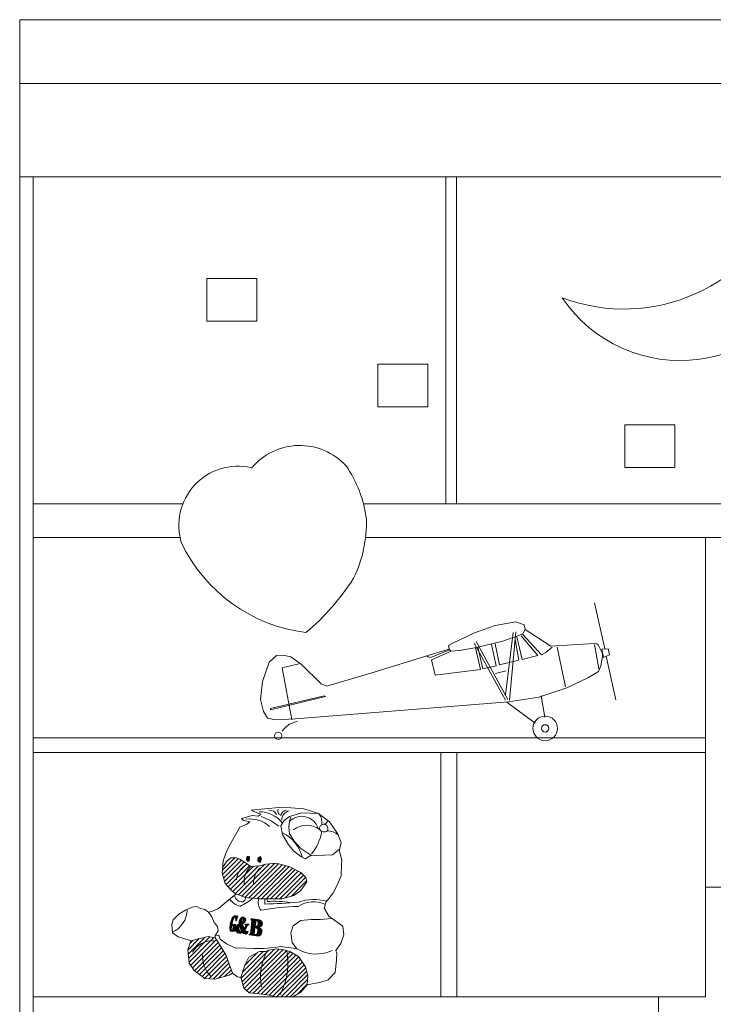
# Model space of a CAD drawing. Units: inches. Extents: x -17 to 1735, y -531 to 60.
# Tile 18 of 27: x 1734.74915 to 1734.79189, y -150.22283 to -150.1622. Entities that reach past the tile are written whole.
import ezdxf

# ---------------------------------------------------------------- set-up
doc = ezdxf.new("R2010")
doc.units = ezdxf.units.IN
doc.header["$MEASUREMENT"] = 0
doc.layers.add('A-FURN', color=242, linetype='Continuous', lineweight=18, true_color=0xcd2027)
pattern_1 = [(45, (83.2096205, 66.2048545), (-0.00092807765, 0.00092807765), [])]

# ---------------------------------------------------------------- blocks, each defined once
blk = doc.blocks.new('childrens_room_2')
h = blk.add_hatch()
h.set_pattern_fill('ANSI31', color=256, scale=0.04, style=0)
h.set_pattern_definition([(45, (82.705578, 65.006513), (-0.0035355339, 0.0035355339), [])])
h.paths.add_polyline_path([(72.4235, 54.2103), (72.4101, 54.2094), (72.3996, 54.2165), (72.3931, 54.2205), (72.3877, 54.2227), (72.3787, 54.2227), (72.3724, 54.2176), (72.3662, 54.2083), (72.3653, 54.1987), (72.3698, 54.1825), (72.3793, 54.1724), (72.3866, 54.1657), (72.3928, 54.1641), (72.4008, 54.1607), (72.4243, 54.1584), (72.4586, 54.1587), (72.4773, 54.1638), (72.4878, 54.1712), (72.4977, 54.1853), (72.496, 54.1918), (72.4884, 54.1998), (72.4711, 54.2088), (72.4501, 54.2142), (72.4337, 54.2131)])
h.paths.add_polyline_path([(72.3715, 54.0699), (72.3593, 54.0898), (72.3544, 54.0977), (72.3431, 54.0995), (72.3306, 54.0968), (72.316, 54.0928), (72.3115, 54.0788), (72.3137, 54.0581), (72.3216, 54.0463), (72.3379, 54.034), (72.3536, 54.0329), (72.376, 54.039), (72.3816, 54.0424)])
h.paths.add_polyline_path([(72.4331, 54.076), (72.4234, 54.0763), (72.4069, 54.0675), (72.4005, 54.055), (72.3945, 54.0357), (72.399, 54.0189), (72.4074, 54.0116), (72.4281, 54.0093), (72.4393, 54.0077), (72.4517, 54.0049), (72.4651, 54.006), (72.4758, 54.0054), (72.4881, 54.0127), (72.4982, 54.0239), (72.4994, 54.0382), (72.4957, 54.0522), (72.485, 54.0681), (72.4713, 54.076), (72.4615, 54.0791), (72.4508, 54.0803), (72.4383, 54.0782)])
h = blk.add_hatch()
h.set_pattern_fill('ANSI31', color=256, scale=0.00525, style=0)
h.set_pattern_definition([(45, (83.20962045, 66.20485446), (-0.000464038825, 0.000464038825), [])])
h.paths.add_polyline_path([(72.4073, 54.2255), (72.4082, 54.2215), (72.4077, 54.2173), (72.4046, 54.2175), (72.4035, 54.2199), (72.4038, 54.2239), (72.4048, 54.2249)])
edge = h.paths.add_edge_path()
edge.add_line((72.4254, 54.2248), (72.4267, 54.2217))
edge.add_line((72.4267, 54.2217), (72.4259, 54.2175))
edge.add_line((72.4259, 54.2175), (72.4239, 54.2152))
edge.add_line((72.4239, 54.2152), (72.421, 54.2178))
edge.add_line((72.421, 54.2178), (72.4212, 54.2219))
edge.add_line((72.4212, 54.2219), (72.4231, 54.224))
edge.add_line((72.4231, 54.224), (72.4253, 54.225))
h = blk.add_hatch()
h.set_pattern_fill('ANSI31', color=256, scale=0.0105, style=0)
h.set_pattern_definition(pattern_1)
h.paths.add_polyline_path([(72.3979, 54.1276), (72.3988, 54.1252), (72.3977, 54.1225), (72.3966, 54.1221), (72.3958, 54.1247), (72.3964, 54.1271), (72.3973, 54.1276)], flags=16)
h.paths.add_polyline_path([(72.4015, 54.119), (72.4063, 54.119), (72.4072, 54.1177), (72.4048, 54.1172), (72.403, 54.113), (72.401, 54.111), (72.4019, 54.108), (72.4044, 54.1073), (72.4059, 54.1079), (72.4046, 54.1048), (72.4021, 54.1031), (72.3984, 54.1042), (72.3969, 54.1055), (72.3957, 54.1055), (72.3933, 54.1046), (72.3894, 54.1053), (72.3867, 54.1088), (72.3872, 54.1139), (72.3894, 54.1177), (72.3918, 54.1194), (72.3916, 54.1238), (72.3933, 54.1276), (72.396, 54.1298), (72.3988, 54.1298), (72.4017, 54.1278), (72.4022, 54.1247), (72.4004, 54.1212), (72.3971, 54.1194), (72.3991, 54.1132), (72.3999, 54.1121), (72.4017, 54.1148), (72.4021, 54.1174), (72.4008, 54.1185)])
h.paths.add_polyline_path([(72.3876, 54.1243), (72.3885, 54.1287), (72.3896, 54.132), (72.3882, 54.1313), (72.3869, 54.1322), (72.3852, 54.1325), (72.3809, 54.1291), (72.3776, 54.1199), (72.3774, 54.111), (72.3785, 54.108), (72.381, 54.1075), (72.3854, 54.108), (72.3865, 54.1146), (72.3871, 54.1172), (72.3867, 54.1185), (72.3819, 54.119), (72.3807, 54.1185), (72.3825, 54.1159), (72.3819, 54.1102), (72.3801, 54.1093), (72.3794, 54.1119), (72.3801, 54.1174), (72.3814, 54.1227), (72.3832, 54.1291), (72.3849, 54.1298), (72.3867, 54.1271), (72.3867, 54.1241), (72.3876, 54.1241)])
edge = h.paths.add_edge_path(flags=16)
edge.add_line((72.3924, 54.117), (72.3951, 54.109))
edge.add_line((72.3951, 54.109), (72.3957, 54.108))
edge.add_line((72.3957, 54.108), (72.3935, 54.1075))
edge.add_line((72.3935, 54.1075), (72.3915, 54.1106))
edge.add_line((72.3915, 54.1106), (72.3911, 54.1166))
edge.add_line((72.3911, 54.1166), (72.3923, 54.1171))
h = blk.add_hatch()
h.set_pattern_fill('ANSI31', color=256, scale=0.0105, style=0)
h.set_pattern_definition(pattern_1)
h.paths.add_polyline_path([(72.4118, 54.1249), (72.4103, 54.1262), (72.4104, 54.1272), (72.4131, 54.1271), (72.4234, 54.1257), (72.4267, 54.1243), (72.4282, 54.121), (72.4277, 54.1174), (72.4256, 54.1151), (72.4231, 54.1141), (72.4247, 54.1125), (72.4265, 54.1111), (72.4276, 54.1084), (72.4264, 54.103), (72.4236, 54.1009), (72.4182, 54.1009), (72.4077, 54.1023), (72.4073, 54.1036), (72.4096, 54.1041)])
h.paths.add_polyline_path([(72.4163, 54.1135), (72.4153, 54.1032), (72.4163, 54.1027), (72.4194, 54.1034), (72.4205, 54.1049), (72.4209, 54.1097), (72.4196, 54.113), (72.4181, 54.1138)], flags=16)
edge = h.paths.add_edge_path(flags=16)
edge.add_line((72.4183, 54.1245), (72.4166, 54.1157))
edge.add_line((72.4166, 54.1157), (72.419, 54.1153))
edge.add_line((72.419, 54.1153), (72.4209, 54.1169))
edge.add_line((72.4209, 54.1169), (72.4217, 54.1213))
edge.add_line((72.4217, 54.1213), (72.4207, 54.1241))
edge.add_line((72.4207, 54.1241), (72.4183, 54.1245))
for p, q in [((72.0483, 55.5336), (72.0483, 52.9336)), ((72.0483, 55.5336), (74.0483, 55.5336)), ((72.0483, 55.4336), (74.0483, 55.4336)), ((72.0483, 55.2879), (74.0483, 55.2879)), ((72.0693, 55.2879), (72.0693, 52.9336)), ((72.7152, 55.2879), (72.7152, 54.7763)), ((72.7319, 55.2879), (72.7319, 54.7763)), ((72.3037, 54.7763), (72.0693, 54.7763)), ((73.6316, 54.7763), (72.5863, 54.7763)), ((72.0693, 54.7238), (72.2994, 54.7238)), ((72.5896, 54.7238), (73.6316, 54.7238)), ((73.1216, 54.7238), (73.1216, 54.0054)), ((72.948, 54.6216), (72.9639, 54.5495)), ((72.7926, 54.5862), (72.7599, 54.5744)), ((72.8248, 54.5919), (72.7926, 54.5862)), ((72.8378, 54.5872), (72.8248, 54.5919)), ((72.8353, 54.5728), (72.8396, 54.5797)), ((72.8396, 54.5797), (72.8378, 54.5872)), ((72.8794, 54.5537), (72.8396, 54.5797)), ((72.7599, 54.5744), (72.7262, 54.5584)), ((72.8353, 54.5728), (72.8045, 54.5614)), ((72.8209, 54.5752), (72.8088, 54.4775)), ((72.8246, 54.5761), (72.8148, 54.4691)), ((72.8237, 54.5641), (72.8294, 54.5318)), ((72.835, 54.5332), (72.8264, 54.5686)), ((72.833, 54.5702), (72.8592, 54.539)), ((72.8648, 54.5403), (72.8353, 54.5728)), ((72.7205, 54.5491), (72.6855, 54.5387)), ((72.7208, 54.5481), (72.692, 54.5363)), ((72.7262, 54.5584), (72.7192, 54.5547)), ((72.7192, 54.5547), (72.7205, 54.5491)), ((72.7233, 54.5458), (72.7205, 54.5491)), ((72.7368, 54.5471), (72.7233, 54.5458)), ((72.7634, 54.5515), (72.7368, 54.5471)), ((72.7597, 54.5585), (72.8088, 54.4696)), ((72.7616, 54.5511), (72.7696, 54.5175)), ((72.763, 54.5613), (72.8125, 54.4705)), ((72.8045, 54.5614), (72.7634, 54.5515)), ((72.7733, 54.5183), (72.7653, 54.552)), ((72.787, 54.5562), (72.7939, 54.5233)), ((72.7995, 54.5246), (72.7926, 54.5576)), ((72.8817, 54.5523), (72.8719, 54.544)), ((72.9474, 54.5582), (72.8794, 54.5537)), ((72.9026, 54.4902), (72.8896, 54.5522)), ((72.9516, 54.5573), (72.9474, 54.5582)), ((72.955, 54.5186), (72.9479, 54.5564)), ((72.9539, 54.5558), (72.9516, 54.5573)), ((72.9599, 54.5435), (72.9539, 54.5558)), ((72.9693, 54.5496), (72.9595, 54.5493)), ((72.9621, 54.5362), (72.9595, 54.5493)), ((72.9715, 54.5403), (72.9693, 54.5496)), ((72.4502, 54.5394), (72.439, 54.5288)), ((72.46, 54.5398), (72.4502, 54.5394)), ((72.4726, 54.5369), (72.46, 54.5398)), ((72.4892, 54.5251), (72.4726, 54.5369)), ((72.6855, 54.5387), (72.6047, 54.5134)), ((72.6878, 54.5373), (72.6858, 54.5388)), ((72.692, 54.5363), (72.6878, 54.5373)), ((72.6929, 54.5326), (72.7224, 54.5456)), ((72.6987, 54.5083), (72.6929, 54.5326)), ((72.8294, 54.5318), (72.7995, 54.5246)), ((72.8592, 54.539), (72.835, 54.5332)), ((72.8719, 54.544), (72.8648, 54.5403)), ((72.9578, 54.5232), (72.9603, 54.5376)), ((72.9599, 54.5435), (72.9603, 54.5416)), ((72.9603, 54.5376), (72.9603, 54.5416)), ((72.9621, 54.5362), (72.9715, 54.5403)), ((72.9665, 54.5381), (72.9816, 54.4697)), ((72.439, 54.5288), (72.4284, 54.4986)), ((72.4851, 54.5261), (72.4589, 54.5198)), ((72.4589, 54.5198), (72.4745, 54.4386)), ((72.5202, 54.495), (72.4892, 54.5251)), ((72.7696, 54.5175), (72.6987, 54.5083)), ((72.7939, 54.5233), (72.7733, 54.5183)), ((72.954, 54.5144), (72.9578, 54.5232)), ((72.6047, 54.5134), (72.529, 54.4912)), ((72.8096, 54.5152), (72.7928, 54.5112)), ((72.9049, 54.4887), (72.9386, 54.5047)), ((72.9386, 54.5047), (72.954, 54.5144)), ((72.4284, 54.4986), (72.4254, 54.4703)), ((72.529, 54.4912), (72.5202, 54.495)), ((72.861, 54.4742), (72.9049, 54.4887)), ((72.4254, 54.4703), (72.4299, 54.4516)), ((72.5247, 54.4763), (72.4406, 54.4561)), ((72.4411, 54.4543), (72.527, 54.4749)), ((72.527, 54.4749), (72.5247, 54.4763)), ((72.8134, 54.4667), (72.861, 54.4742)), ((72.8645, 54.4761), (72.8705, 54.4429)), ((72.4406, 54.4561), (72.4411, 54.4543)), ((72.4801, 54.44), (72.8134, 54.4667)), ((72.8106, 54.4661), (72.855, 54.4333)), ((72.4299, 54.4516), (72.4363, 54.4413)), ((72.4363, 54.4413), (72.4489, 54.4384)), ((72.4489, 54.4384), (72.4801, 54.44)), ((72.4637, 54.4261), (72.459, 54.421)), ((72.4702, 54.4317), (72.4637, 54.4261)), ((72.4829, 54.4367), (72.4702, 54.4317)), ((72.0693, 54.4104), (73.1216, 54.4104)), ((72.0693, 54.3874), (73.1216, 54.3874)), ((72.7074, 54.0054), (72.7074, 54.3874)), ((72.7323, 54.0054), (72.7323, 54.3874)), ((73.8625, 54.1771), (73.1216, 54.1771)), ((72.0693, 54.0054), (73.1216, 54.0054)), ((73.0483, 52.9336), (73.0483, 54.0054))]:
    blk.add_line(p, q)
for points in [[(72.3413, 55.1291), (72.4195, 55.1291), (72.4195, 55.062), (72.3413, 55.062)], [(72.609, 54.995), (72.6872, 54.995), (72.6872, 54.928), (72.609, 54.928)], [(72.9953, 54.9001), (73.0735, 54.9001), (73.0735, 54.8331), (72.9953, 54.8331)]]:
    blk.add_lwpolyline(points, close=True)
for points in [[(72.3866, 54.1657), (72.3726, 54.1545), (72.3597, 54.1433), (72.3491, 54.1388), (72.344, 54.1377), (72.3379, 54.1421), (72.3311, 54.1433), (72.3255, 54.1466), (72.3182, 54.1455), (72.3076, 54.141), (72.2975, 54.1349), (72.2885, 54.1259), (72.2863, 54.1186), (72.2874, 54.1057), (72.2964, 54.099), (72.3121, 54.0945), (72.316, 54.0928), (72.3115, 54.0788), (72.3137, 54.0581), (72.3216, 54.0463), (72.3379, 54.034), (72.3536, 54.0329), (72.376, 54.039), (72.3816, 54.0424), (72.3894, 54.0368), (72.3945, 54.0357), (72.399, 54.0189), (72.4074, 54.0116), (72.4281, 54.0093), (72.4393, 54.0077), (72.4517, 54.0049), (72.4651, 54.006), (72.4758, 54.0054), (72.4881, 54.0127), (72.4982, 54.0239), (72.5195, 54.0284), (72.5313, 54.0318), (72.542, 54.0435), (72.5442, 54.0626), (72.5448, 54.0738), (72.5431, 54.0777), (72.5509, 54.0889), (72.5554, 54.1024), (72.5543, 54.1158), (72.5414, 54.1248), (72.5319, 54.1315), (72.5251, 54.1438), (72.5279, 54.1539), (72.5386, 54.1668), (72.5453, 54.1802), (72.5515, 54.1948), (72.552, 54.2111), (72.5526, 54.2195), (72.5487, 54.2324), (72.5487, 54.2363), (72.5515, 54.2464), (72.547, 54.2587), (72.5436, 54.2637), (72.533, 54.2789), (72.5162, 54.2923), (72.4932, 54.2996), (72.459, 54.3018), (72.4321, 54.2996), (72.4107, 54.2974), (72.4186, 54.2934), (72.4259, 54.2912), (72.422, 54.2878), (72.4124, 54.289), (72.3956, 54.2845), (72.3984, 54.2811), (72.4085, 54.2788), (72.404, 54.2755), (72.3928, 54.2705), (72.3793, 54.2469), (72.3721, 54.2324), (72.367, 54.2178), (72.3653, 54.1987), (72.3698, 54.1825), (72.3793, 54.1724), (72.3866, 54.1657)], [(72.5162, 54.2923), (72.4898, 54.2933), (72.4704, 54.2876), (72.4624, 54.2813), (72.4572, 54.2727), (72.4595, 54.259), (72.4687, 54.2442), (72.4767, 54.2339), (72.4881, 54.2247), (72.495, 54.2213), (72.503, 54.2259), (72.5127, 54.2264), (72.5378, 54.2276), (72.5464, 54.2344), (72.5487, 54.2363)], [(72.5058, 54.226), (72.4881, 54.2373), (72.4784, 54.2482), (72.4704, 54.2602), (72.4698, 54.271), (72.4704, 54.2802), (72.4727, 54.2864)], [(72.4101, 54.2094), (72.3996, 54.2165), (72.3931, 54.2205), (72.3877, 54.2227), (72.3787, 54.2227), (72.3724, 54.2176), (72.3662, 54.2083)], [(72.4073, 54.2255), (72.4082, 54.2215), (72.4077, 54.2173), (72.4046, 54.2175), (72.4035, 54.2199), (72.4038, 54.2239), (72.4048, 54.2249), (72.4073, 54.2255)], [(72.4254, 54.2248), (72.4267, 54.2217), (72.4259, 54.2175), (72.4239, 54.2152), (72.421, 54.2178), (72.4212, 54.2219), (72.4231, 54.224), (72.4253, 54.225)], [(72.4101, 54.2094), (72.4235, 54.2103), (72.4337, 54.2131), (72.4501, 54.2142), (72.4711, 54.2088), (72.4884, 54.1998), (72.496, 54.1918), (72.4977, 54.1853), (72.4878, 54.1712), (72.4773, 54.1638), (72.4586, 54.1587), (72.4243, 54.1584), (72.4008, 54.1607), (72.3928, 54.1641), (72.3866, 54.1657)], [(72.344, 54.1377), (72.3492, 54.1307), (72.3525, 54.1218), (72.358, 54.1151), (72.3589, 54.1087), (72.3544, 54.1014)], [(72.3876, 54.1243), (72.3885, 54.1287), (72.3896, 54.132), (72.3882, 54.1313), (72.3869, 54.1322), (72.3852, 54.1325), (72.3809, 54.1291), (72.3776, 54.1199), (72.3774, 54.111), (72.3785, 54.108), (72.381, 54.1075), (72.3854, 54.108), (72.3865, 54.1146), (72.3871, 54.1172), (72.3867, 54.1185), (72.3819, 54.119), (72.3807, 54.1185), (72.3825, 54.1159), (72.3819, 54.1102), (72.3801, 54.1093), (72.3794, 54.1119), (72.3801, 54.1174), (72.3814, 54.1227), (72.3832, 54.1291), (72.3849, 54.1298), (72.3867, 54.1271), (72.3867, 54.1241), (72.3876, 54.1241), (72.3876, 54.1243)], [(72.4015, 54.119), (72.4063, 54.119), (72.4072, 54.1177), (72.4048, 54.1172), (72.403, 54.113), (72.401, 54.111), (72.4019, 54.108), (72.4044, 54.1073), (72.4059, 54.1079), (72.4046, 54.1048), (72.4021, 54.1031), (72.3984, 54.1042), (72.3969, 54.1055), (72.3957, 54.1055), (72.3933, 54.1046), (72.3894, 54.1053), (72.3867, 54.1088), (72.3872, 54.1139), (72.3894, 54.1177), (72.3918, 54.1194), (72.3916, 54.1238), (72.3933, 54.1276), (72.396, 54.1298), (72.3988, 54.1298), (72.4017, 54.1278), (72.4022, 54.1247), (72.4004, 54.1212), (72.3971, 54.1194), (72.3991, 54.1132), (72.3999, 54.1121), (72.4017, 54.1148), (72.4021, 54.1174), (72.4008, 54.1185), (72.4015, 54.119)], [(72.3924, 54.117), (72.3951, 54.109), (72.3957, 54.108), (72.3935, 54.1075), (72.3915, 54.1106), (72.3911, 54.1166), (72.3923, 54.1171)], [(72.3979, 54.1276), (72.3988, 54.1252), (72.3977, 54.1225), (72.3966, 54.1221), (72.3958, 54.1247), (72.3964, 54.1271), (72.3973, 54.1276), (72.3979, 54.1276)], [(72.4118, 54.1249), (72.4103, 54.1262), (72.4104, 54.1272), (72.4131, 54.1271), (72.4234, 54.1257), (72.4267, 54.1243), (72.4282, 54.121), (72.4277, 54.1174), (72.4256, 54.1151), (72.4231, 54.1141), (72.4247, 54.1125), (72.4265, 54.1111), (72.4276, 54.1084), (72.4264, 54.103), (72.4236, 54.1009), (72.4182, 54.1009), (72.4077, 54.1023), (72.4073, 54.1036), (72.4096, 54.1041), (72.4118, 54.1249)], [(72.4183, 54.1245), (72.4166, 54.1157), (72.419, 54.1153), (72.4209, 54.1169), (72.4217, 54.1213), (72.4207, 54.1241), (72.4183, 54.1245)], [(72.5366, 54.1281), (72.5192, 54.1264), (72.5043, 54.1261), (72.4881, 54.1249), (72.4765, 54.1163), (72.4725, 54.1056), (72.4749, 54.0901), (72.4823, 54.0806), (72.4734, 54.0818), (72.4566, 54.084)], [(72.316, 54.0928), (72.3306, 54.0968), (72.3431, 54.0995), (72.3544, 54.0977)], [(72.3544, 54.0977), (72.3544, 54.1014), (72.3599, 54.1017)], [(72.3599, 54.1017), (72.362, 54.0953), (72.3718, 54.0882), (72.3867, 54.0815), (72.3925, 54.0818), (72.4142, 54.0809), (72.431, 54.0809), (72.4508, 54.0828), (72.4566, 54.084)], [(72.4163, 54.1135), (72.4153, 54.1032), (72.4163, 54.1027), (72.4194, 54.1034), (72.4205, 54.1049), (72.4209, 54.1097), (72.4196, 54.113), (72.4181, 54.1138), (72.4163, 54.1135)], [(72.3816, 54.0424), (72.3715, 54.0699), (72.3593, 54.0898), (72.3544, 54.0977)], [(72.4982, 54.0239), (72.4994, 54.0382), (72.4957, 54.0522), (72.485, 54.0681), (72.4713, 54.076), (72.4615, 54.0791), (72.4508, 54.0803), (72.4383, 54.0782), (72.4331, 54.076), (72.4234, 54.0763), (72.4069, 54.0675), (72.4005, 54.055), (72.3945, 54.0357)]]:
    blk.add_lwpolyline(points)
for centre, radius in [((72.8708, 54.4252), 0.0192), ((72.8708, 54.4252), 0.00576), ((72.4528, 54.4136), 0.00576)]:
    blk.add_circle(centre, radius)
for centre, radius, start, end in [((72.9941, 55.3549), 0.2738, 249.3531, 339.0618), ((73.0818, 55.2225), 0.222, 213.9015, 341.8175), ((72.4867, 54.7693), 0.0984, 42.595, 140.2536), ((72.3899, 54.7429), 0.0925, 77.2464, 197.7091), ((72.3988, 54.7269), 0.1939, 7.6537, 34.2134), ((72.3899, 54.748), 0.2012, 334.0468, 1.3639), ((72.5266, 54.8228), 0.2495, 205.6711, 263.0236), ((72.2561, 54.8613), 0.3736, 310.0169, 327.3881), ((72.4234, 54.2488), 0.046, 37.8322, 90.3836), ((72.3965, 54.2013), 0.091, 51.0314, 70.9793), ((72.4391, 54.284), 0.0131, 30.153, 92.9921), ((72.4607, 54.2966), 0.00841, 163.2453, 226.426), ((72.4674, 54.2863), 0.011, 101.4803, 166.7726), ((72.4736, 54.2816), 0.0152, 103.9194, 180.1604), ((72.4897, 54.2607), 0.027, 17.9097, 136.1322), ((72.5003, 54.2787), 0.0211, 348.7721, 36.4235), ((72.409, 54.2387), 0.0449, 47.4427, 98.5655), ((72.4975, 54.241), 0.0329, 52.0739, 129.3049), ((72.5242, 54.2687), 0.00663, 325.8624, 195.236), ((72.5214, 54.2829), 0.0088, 295.5344, 349.1087), ((72.4339, 54.209), 0.0587, 13.7841, 64.1856), ((72.4439, 54.2787), 0.0788, 320.8041, 349.2846), ((72.5247, 54.2715), 0.00821, 213.2814, 307.817), ((72.5293, 54.2375), 0.0275, 49.7311, 89.2181), ((72.4171, 54.1858), 0.0297, 114.2463, 175.5155), ((72.4349, 54.184), 0.0355, 134.2978, 186.5108), ((72.4466, 54.1827), 0.0325, 130.6295, 181.4181), ((72.3963, 54.1658), 0.012, 189.8899, 275.0416), ((72.3998, 54.1727), 0.0267, 212.7395, 254.9049), ((72.3518, 54.2366), 0.0987, 294.607, 308.8483), ((72.3928, 54.163), 0.0102, 296.1834, 345.8834), ((72.4415, 54.153), 0.0198, 162.6389, 218.8134), ((72.4858, 53.84), 0.3066, 90.3272, 101.242), ((72.4096, 55.0164), 0.8663, 271.4495, 274.9615), ((72.4071, 54.1543), 0.025, 350.8842, 9.5622), ((72.4244, 54.1546), 0.0116, 358.7797, 19.7643), ((72.4476, 54.0284), 0.1264, 78.6572, 95.2788), ((72.5084, 54.1102), 0.0438, 65.1368, 123.7987), ((72.5088, 54.0869), 0.0707, 73.6731, 110.0465), ((72.2712, 54.1421), 0.0392, 294.5591, 358.2889), ((72.349, 54.0584), 0.0345, 85.1231, 150.4946), ((72.3816, 54.0704), 0.0475, 177.9767, 223.7147), ((72.5074, 54.0367), 0.0823, 150.5878, 191.3286), ((72.362, 54.058), 0.1062, 332.2749, 10.6031), ((72.5122, 54.1302), 0.058, 238.8884, 295.4462)]:
    blk.add_arc(centre, radius, start, end)

msp = doc.modelspace()

# ---------------------------------------------------------------- block references
at = {"layer": 'A-FURN', "xscale": 0.0393700787401575, "yscale": 0.0393700787401575, "zscale": 0.0393700787401575}
msp.add_blockref('childrens_room_2', (1731.912601, -152.348565), dxfattribs=at)

doc.saveas('drawing.dxf')
